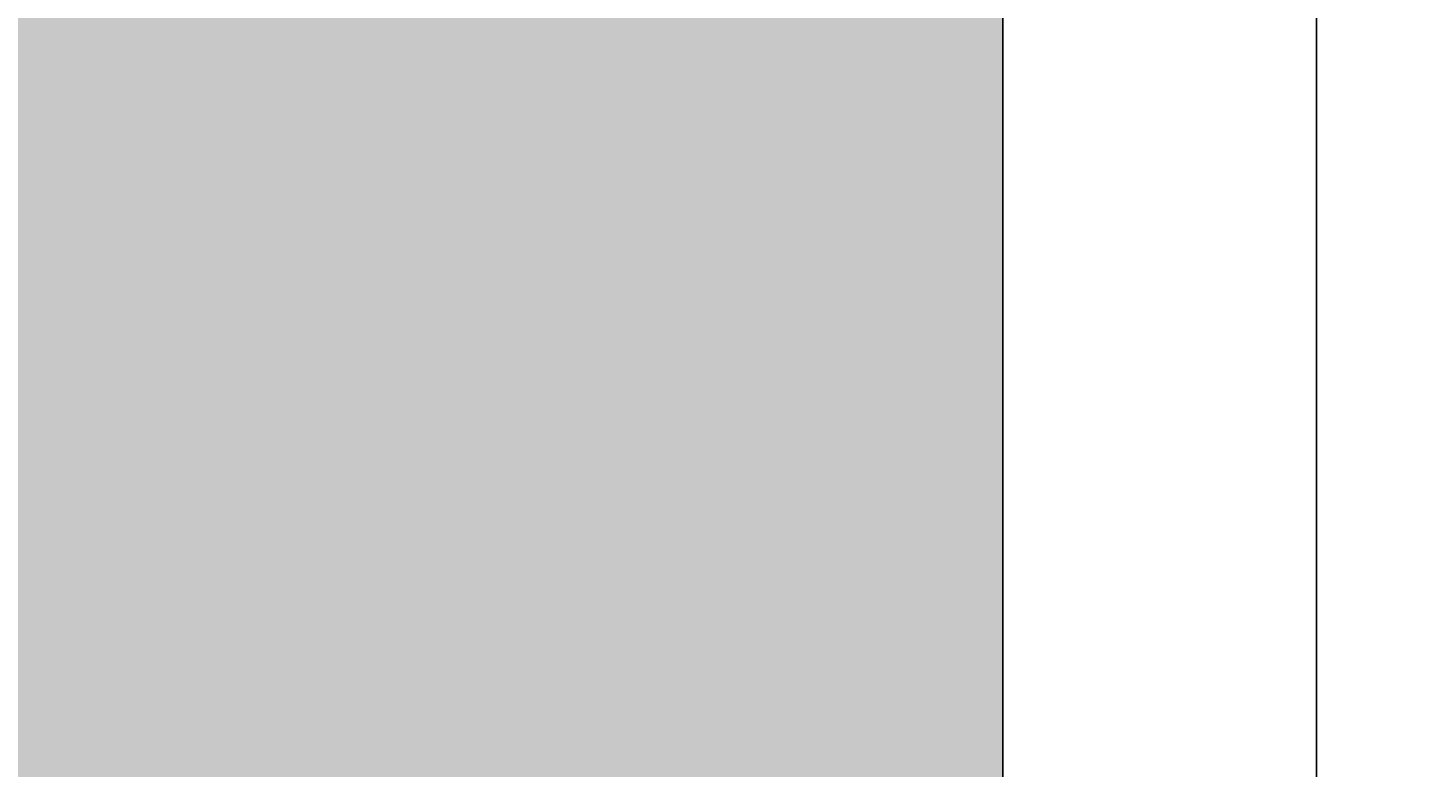
# Model space of a CAD drawing. Units: inches. Extents: x 84 to 1044, y -280 to 906.
# Tile 45 of 105: x 955 to 995, y -88 to -66. Entities that reach past the tile are written whole.
import ezdxf

# ---------------------------------------------------------------- set-up
doc = ezdxf.new("R2010")
doc.units = ezdxf.units.IN
doc.layers.add('A-ANNO-DIMS', color=2, linetype='Continuous', lineweight=18)
doc.layers.add('C-PROP', color=7, linetype='Continuous', lineweight=25)
doc.layers.add('L-PLNT-PATT', color=9, linetype='Continuous', lineweight=9, true_color=0xafd9aa)
doc.styles.get("Standard").update_dxf_attribs({"font": 'arial.ttf'})
doc.dimstyles.get("Standard").update_dxf_attribs({"dimtxt": 0.18, "dimasz": 0.18, "dimexe": 0.18, "dimexo": 0.0625, "dimgap": 0.09, "dimtad": 0, "dimtih": 1, "dimtoh": 1, "dimdec": 4, "dimzin": 0, "dimdsep": 46, "dimtxsty": 'Standard', "dimcen": 0.09, "dimadec": 0, "dimazin": 0, "dimtfac": 1, "dimtdec": 4, "dimtofl": 0, "dimtmove": 0, "dimatfit": 3, "dimfxl": 1, "dimtolj": 1, "dimtzin": 0, "dimarcsym": 0})

# ---------------------------------------------------------------- blocks, each defined once
blk = doc.blocks.new('*D70')
at = {"layer": 'A-ANNO-DIMS', "color": 0, "lineweight": -2, "transparency": 16777216}
for p, q in [((983.136, -64.88), (1043.768, -64.88)), ((1043.588, -65.06), (1043.588, -93.198)), ((1043.588, -121.7), (1043.588, -93.561)), ((992.136, -121.88), (1043.768, -121.88))]:
    blk.add_line(p, q, dxfattribs=at)
at = {"layer": 'A-ANNO-DIMS', "color": 0, "transparency": 16777216}
for points in [[(1043.558, -65.06), (1043.618, -65.06), (1043.588, -64.88)], [(1043.558, -121.7), (1043.618, -121.7), (1043.588, -121.88)]]:
    blk.add_solid(points, dxfattribs=at)
at = {"layer": 'Defpoints', "color": 0, "transparency": 16777216}
for p in [(983.074, -64.88), (1043.588, -64.88), (992.074, -121.88)]:
    blk.add_point(p, dxfattribs=at)
at = {"layer": 'A-ANNO-DIMS', "color": 0, "transparency": 16777216, "insert": (1043.588, -93.38), "char_height": 0.18, "attachment_point": 5}
blk.add_mtext('\\A1;57', dxfattribs=at)

msp = doc.modelspace()

# ---------------------------------------------------------------- hatches: boundary and pattern name
at = {"layer": 'L-PLNT-PATT', "transparency": 33554597}
h = msp.add_hatch(color=256, dxfattribs=at)
h.dxf.hatch_style = 1
h.paths.add_polyline_path([(791.074, 31.12), (791.074, 91.12), (743.074, 91.12), (674.074, 91.12), (674.074, 31.12), (650.074, 31.12), (650.074, -112.88), (983.074, -112.88), (983.074, -64.88), (791.074, -64.88)])

# ---------------------------------------------------------------- linework, layer by layer
at = {"layer": 'C-PROP'}
for points in [[(143.179, -121.88), (134.179, -121.88), (134.179, 856.12), (992.074, 856.12), (992.074, -121.88), (624.574, -121.88)], [(143.179, -112.88), (143.179, 847.12), (983.074, 847.12), (983.074, -112.88), (624.574, -112.88)]]:
    msp.add_lwpolyline(points, dxfattribs=at)

# ---------------------------------------------------------------- dimensions: what is measured, and where the dimension line sits
at = {"layer": 'A-ANNO-DIMS'}
dim = msp.add_linear_dim(base=(1043.588, -64.88), p1=(992.074, -121.88), p2=(983.074, -64.88), angle=90, dimstyle='Standard', override={"dimdec": 0, "dimlfac": 1, "dimrnd": 0, "dimzin": 0, "dimdsep": 46, "dimlunit": 2}, dxfattribs=at)
dim.commit()
dim.dimension.update_dxf_attribs({"geometry": '*D70', "text_midpoint": (1043.588, -93.38)})

doc.saveas('drawing.dxf')
